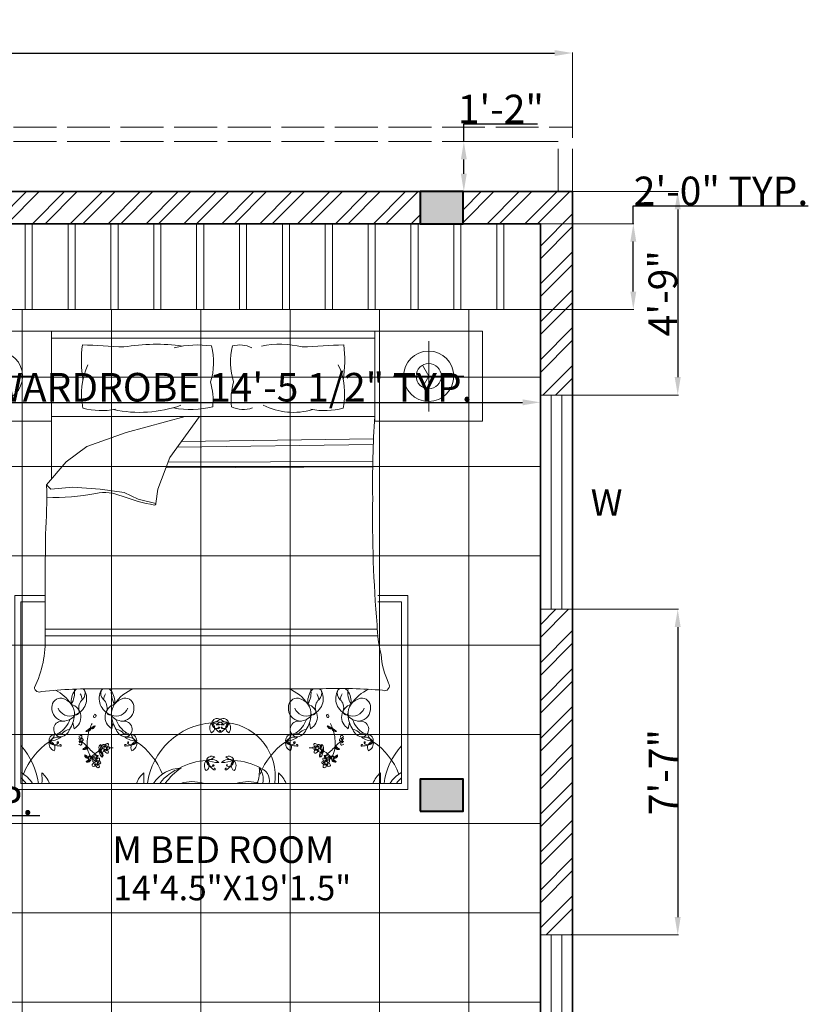
# Model space of a CAD drawing. Units: inches. Extents: x 351 to 1738, y -265 to 286.
# Tile 7 of 38: x 759 to 980, y 10 to 286. Entities that reach past the tile are written whole.
import ezdxf

# ---------------------------------------------------------------- set-up
doc = ezdxf.new("R2010")
doc.units = ezdxf.units.IN
doc.header["$MEASUREMENT"] = 0
doc.linetypes.add('ACAD_ISO02W100', pattern=[15, 12, -3])
for name, color, linetype, lineweight in [('A-ANNO-DIMS', 2, 'Continuous', 18), ('A-ANNO-SYMB', 7, 'Continuous', 18), ('A-AREA-IDEN', 7, 'Continuous', 18), ('A-COLS', 7, 'Continuous', 40), ('A-COLS-PATT', 6, 'Continuous', 13), ('A-FLOR-CASE', 9, 'Continuous', 18), ('A-FLOR-OVHD', 1, 'ACAD_ISO02W100', 18), ('A-FLOR-PATT', 9, 'Continuous', 9), ('A-FURN', 18, 'Continuous', 13), ('A-GLAZ', 4, 'Continuous', 18), ('A-WALL', 7, 'Continuous', 35), ('A-WALL-PATT', 152, 'Continuous', 13)]:
    doc.layers.add(name, color=color, linetype=linetype, lineweight=lineweight)
doc.styles.add('Annotative', font='arial.ttf')
doc.styles.get("Standard").update_dxf_attribs({"font": 'arial.ttf'})
doc.dimstyles.get("Standard").update_dxf_attribs({"dimtxt": 8, "dimasz": 5, "dimexe": 0.18, "dimexo": 0.0625, "dimgap": 0.09, "dimtad": 1, "dimtoh": 1, "dimzin": 0, "dimdsep": 46, "dimlunit": 4, "dimtxsty": 'Standard', "dimcen": 0, "dimclre": 256, "dimadec": 0, "dimazin": 0, "dimtfac": 1, "dimtofl": 0, "dimtmove": 0, "dimatfit": 3, "dimfxl": 1, "dimtolj": 1, "dimtzin": 0, "dimlwe": -1, "dimarcsym": 0})

# ---------------------------------------------------------------- blocks, each defined once
blk = doc.blocks.new('*D2')
at = {"layer": 'A-ANNO-DIMS', "color": 0, "transparency": 16777216}
for p, q in [((382.16, 256.03), (382.16, 276.92)), ((914.16, 256.03), (914.16, 276.92))]:
    blk.add_line(p, q, dxfattribs=at)
at = {"layer": 'A-ANNO-DIMS', "color": 0, "lineweight": -2, "transparency": 16777216}
blk.add_line((387.16, 276.74), (909.16, 276.74), dxfattribs=at)
at = {"layer": 'A-ANNO-DIMS', "color": 0, "transparency": 16777216}
for points in [[(387.16, 277.57), (387.16, 275.91), (382.16, 276.74)], [(909.16, 277.57), (909.16, 275.91), (914.16, 276.74)]]:
    blk.add_solid(points, dxfattribs=at)
at = {"layer": 'Defpoints', "color": 0, "transparency": 16777216}
for p in [(914.16, 276.74), (382.16, 255.96), (914.16, 255.96)]:
    blk.add_point(p, dxfattribs=at)
at = {"layer": 'A-ANNO-DIMS', "color": 0, "transparency": 16777216, "insert": (648.16, 280.83), "char_height": 8, "attachment_point": 5}
blk.add_mtext('\\A1;44\'-4"', dxfattribs=at)
blk = doc.blocks.new('*D4')
at = {"layer": 'A-ANNO-DIMS', "color": 0, "lineweight": -2, "transparency": 16777216}
for p, q in [((883.73, 251.96), (883.73, 256.96)), ((883.73, 256.96), (904.33, 256.96)), ((883.73, 242.96), (883.73, 246.96))]:
    blk.add_line(p, q, dxfattribs=at)
at = {"layer": 'A-ANNO-DIMS', "color": 0, "transparency": 16777216}
for p, q in [((910.09, 251.96), (883.55, 251.96)), ((910.09, 237.96), (883.55, 237.96))]:
    blk.add_line(p, q, dxfattribs=at)
for points in [[(882.9, 246.96), (884.56, 246.96), (883.73, 251.96)], [(882.9, 242.96), (884.56, 242.96), (883.73, 237.96)]]:
    blk.add_solid(points, dxfattribs=at)
at = {"layer": 'Defpoints', "color": 0, "transparency": 16777216}
for p in [(883.73, 251.96), (910.16, 251.96), (910.16, 237.96)]:
    blk.add_point(p, dxfattribs=at)
at = {"layer": 'A-ANNO-DIMS', "color": 0, "transparency": 16777216, "insert": (894.08, 261.07), "char_height": 8, "attachment_point": 5}
blk.add_mtext('\\A1;1\'-2"', dxfattribs=at)
blk = doc.blocks.new('BED-DOUBLE-W-NIGHTSTANDS')
for p, q in [((30.18, 128.33), (30.18, 86.91)), ((15.09, 105.9), (15.09, 125.61)), ((120.72, 126.39), (30.18, 126.39)), ((135.81, 105.9), (135.81, 125.61)), ((24.95, 115.76), (5.23, 115.76)), ((125.95, 115.76), (145.67, 115.76)), ((30.18, 104.48), (120.72, 104.48)), ((120.26, 96.67), (65.46, 95.89)), ((120.32, 98.22), (66.59, 97.46)), ((120.18, 91.92), (62.88, 91.69)), ((120.19, 90.37), (62.29, 90.13)), ((121.41, 44.95), (28.44, 44.95)), ((121.55, 43.07), (28.44, 43.07)), ((106.08, 28.24), (44.82, 28.24)), ((36.54, 17.05), (36.2, 18.75)), ((47.08, 17.05), (47.42, 18.75)), ((102.76, 17.05), (102.43, 18.75)), ((113.31, 17.05), (113.64, 18.75))]:
    blk.add_line(p, q)
for points in [[(30.18, 103.18), (0, 103.18), (0, 128.33), (150.9, 128.33), (150.9, 103.18), (120.72, 103.18), (120.72, 128.33)], [(16.85, 112.71), (15.09, 115.76), (16.85, 118.81)], [(134.05, 118.81), (135.81, 115.76), (134.05, 112.71)], [(71.64, 104.48), (63.37, 92.97), (60, 84.12), (59.39, 80.15), (54.5, 81.37), (50.53, 83.2), (43.81, 84.12), (36.16, 84.73), (30.05, 84.12), (28.83, 85.34), (34.33, 91.75), (40.14, 96.03), (51.14, 100), (67.6, 104.48)], [(121.56, 54.36), (129.93, 54.36), (129.93, 0), (19.92, 0), (19.92, 54.36), (28.45, 54.36)], [(28.45, 52.61), (21.67, 52.61), (21.67, 1.75), (128.18, 1.75), (128.18, 52.61), (121.53, 52.61)]]:
    blk.add_lwpolyline(points)
for points in [[(38.85, 124.57, 0.074897), (39.03, 114.71, -0.472817)], [(74.74, 114.16, 0.14099), (75.04, 124.22, 0.235245)], [(81.19, 114.16, -0.14099), (80.89, 124.22, -0.235245)], [(112.05, 124.57, -0.074897), (111.87, 114.71, 0.472817)], [(28.51, 71.52, 0.001242), (28.44, 42.89, -0.127202), (25.42, 28.62)], [(121.36, 46.14, 0.056112), (122.46, 37.83, 0.095341), (124.58, 29.84)]]:
    blk.add_lwpolyline(points, format="xyb")
for centre, radius in [((15.09, 115.76), 7.04), ((135.81, 115.76), 7.04), ((15.09, 115.76), 3.52), ((135.81, 115.76), 3.52), ((45.25, 11.58), 0.384), ((104.59, 11.58), 0.384), ((42.74, 7.53), 0.384), ((107.11, 7.53), 0.384)]:
    blk.add_circle(centre, radius)
for centre, radius, start, end in [((122.02, 1560.65), 1438.48, 266.68521, 267.14978), ((59.52, 69.97), 54.73, 82.2196, 99.497), ((71.08, 97.62), 26.89, 81.5249, 103.96), ((82.96, 117.05), 7.46, 63.3437, 106.1026), ((94.14, 98.17), 26.53, 76.3427, 101.1841), ((28.88, 1560.65), 1438.48, 272.85022, 273.31479), ((58.07, 110.76), 19.45, 155.1316, 191.7583), ((92.83, 110.76), 19.45, 348.2417, 24.8684), ((56.95, 109.12), 18.49, 354.0129, 15.8293), ((98.98, 109.12), 18.49, 164.1707, 185.9871), ((54.88, 140.71), 35.07, 258.0397, 289.2615), ((97.94, 124.85), 19.21, 243.8761, 286.1746), ((44.23, 126.34), 20.22, 255.1039, 281.0369), ((69.08, 133.05), 26.61, 259.8617, 283.6238), ((83.97, 114.44), 8, 245.0183, 288.5407), ((106.67, 126.34), 20.22, 258.9631, 284.8961), ((391.24, 86.04), 271.14, 176.1, 180.9282), ((-109.53, 81.59), 138.41, 355.8294, 1.553), ((31.41, 138.78), 56.95, 267.4519, 281.3392), ((45.02, 70.89), 12.28, 66.2616, 101.3392), ((69.87, 137.17), 58.52, 250.1194, 259.3383), ((59.05, 80.02), 0.364, 268.8623, 19.7536), ((473.78, 76.18), 353.69, 179.1145, 184.8735), ((26.8, 28.72), 1.39, 183.98, 297.3412), ((43.02, -128.84), 157.09, 89.3433, 95.6887), ((26.22, 17.62), 11.42, 33.6671, 63.2997), ((41.52, 24.41), 5.82, 145.785, 184.7304), ((30.41, 27.13), 6.25, 328.8218, 9.1554), ((38.15, 26.57), 1.82, 120.0293, 142.325), ((35.25, 25.5), 4.81, 289.2822, 29.1751), ((37.38, 26.93), 2.26, 311.5653, 23.8354), ((38.15, 26.57), 1.82, 44.4517, 63.558), ((48.37, 25.5), 4.81, 150.8249, 250.7178), ((46.24, 26.93), 2.26, 156.1646, 228.4347), ((45.47, 26.57), 1.82, 113.229, 135.5483), ((45.47, 26.57), 1.82, 37.675, 66.7144), ((42.1, 24.41), 5.82, 355.2696, 34.215), ((53.21, 27.13), 6.25, 169.7133, 211.1782), ((57.4, 17.62), 11.42, 111.4941, 146.3329), ((92.44, 17.62), 11.42, 33.6671, 68.5059), ((107.75, 24.41), 5.82, 145.785, 184.7304), ((96.63, 27.13), 6.25, 328.8218, 10.2867), ((104.38, 26.57), 1.82, 113.2856, 142.325), ((101.48, 25.5), 4.81, 289.2822, 29.1751), ((104.38, 26.57), 1.82, 44.4517, 66.7144), ((103.61, 26.93), 2.26, 311.5653, 23.8354), ((110.71, -118.52), 146.84, 85.2402, 91.8035), ((114.6, 25.5), 4.81, 150.8249, 250.7178), ((112.47, 26.93), 2.26, 156.1646, 228.4347), ((111.7, 26.57), 1.82, 106.6343, 135.5483), ((111.7, 26.57), 1.82, 37.675, 72.5814), ((108.32, 24.41), 5.82, 355.2696, 34.215), ((119.44, 27.13), 6.25, 169.249, 211.1782), ((123.63, 17.62), 11.42, 113.6453, 146.3329), ((123.44, 29.07), 1.38, 246.5219, 33.8264), ((32.87, 23.1), 2.55, 84.4856, 181.0538), ((32.09, 21.21), 4.54, 355.2933, 76.921), ((40.93, 22.93), 3.09, 131.5653, 195.1471), ((34.52, 24.63), 4.34, 7.436, 29.9149), ((42.69, 22.93), 3.09, 344.8529, 48.4347), ((49.1, 24.63), 4.34, 150.0851, 172.564), ((51.53, 21.21), 4.54, 103.079, 184.7067), ((50.75, 23.1), 2.55, 358.9462, 95.5144), ((99.1, 23.1), 2.55, 84.4856, 181.0538), ((98.32, 21.21), 4.54, 355.2933, 76.921), ((107.16, 22.93), 3.09, 131.5653, 195.1471), ((100.75, 24.63), 4.34, 7.436, 29.9149), ((108.92, 22.93), 3.09, 344.8529, 48.4347), ((115.33, 24.63), 4.34, 150.0851, 172.564), ((117.76, 21.21), 4.54, 103.079, 184.7067), ((116.98, 23.1), 2.55, 358.9462, 95.5144), ((33.91, 22.74), 3.61, 174.9449, 262.8857), ((35.33, 24.1), 3.5, 201.5819, 291.4221), ((34.67, 20.3), 3.75, 299.9085, 73.1337), ((37.04, 21.88), 0.937, 257.3041, 15.1471), ((48.95, 20.3), 3.75, 106.8663, 240.0915), ((46.58, 21.88), 0.937, 164.8529, 282.6959), ((48.29, 24.1), 3.5, 248.5779, 338.4181), ((49.7, 22.74), 3.61, 277.1143, 5.0551), ((100.14, 22.74), 3.61, 174.9449, 262.8857), ((101.56, 24.1), 3.5, 201.5819, 291.4221), ((100.89, 20.3), 3.75, 299.9085, 73.1337), ((103.27, 21.88), 0.937, 257.3041, 15.1471), ((115.18, 20.3), 3.75, 106.8663, 240.0915), ((112.81, 21.88), 0.937, 164.8529, 282.6959), ((114.52, 24.1), 3.5, 248.5779, 338.4181), ((115.93, 22.74), 3.61, 277.1143, 5.0551), ((28.59, 21.91), 7.12, 301.2614, 341.7045), ((33.29, 23.54), 4.38, 272.3591, 324.0401), ((28.53, 21.34), 8.1, 326.2883, 356.5076), ((41.52, 24.41), 5.82, 212.7011, 216.3445), ((42.24, 20.46), 0.291, 102.7051, 280.4384), ((42.21, 20.63), 0.473, 280.4384, 100.4136), ((42.1, 24.41), 5.82, 323.6555, 327.2989), ((50.33, 23.54), 4.38, 215.9599, 267.6409), ((55.09, 21.34), 8.1, 183.4924, 213.7117), ((55.02, 21.91), 7.12, 198.2955, 238.7386), ((76.66, 18.28), 1.63, 63.0274, 163.8037), ((75, 22.1), 3.37, 271.4585, 315.3727), ((78.22, 18.28), 1.63, 16.1963, 116.9726), ((79.87, 22.1), 3.37, 224.6273, 268.5415), ((94.82, 21.91), 7.12, 301.2614, 341.7045), ((99.52, 23.54), 4.38, 272.3591, 324.0401), ((94.76, 21.34), 8.1, 326.2883, 356.5076), ((107.75, 24.41), 5.82, 212.7011, 216.3445), ((107.64, 20.63), 0.473, 79.5864, 259.5616), ((107.6, 20.46), 0.291, 259.5616, 77.2949), ((108.32, 24.41), 5.82, 323.6555, 327.2989), ((116.56, 23.54), 4.38, 215.9599, 267.6409), ((121.32, 21.34), 8.1, 183.4924, 213.7117), ((121.25, 21.91), 7.12, 198.2955, 238.7386), ((33.08, 16.92), 2.26, 80.264, 250.8688), ((32.54, 17.61), 2.83, 265.969, 344.3045), ((35.59, 13.85), 3.01, 96.1662, 141.5825), ((40.58, 15.96), 0.792, 101.3256, 154.4621), ((39.44, 18.65), 2.39, 280.2588, 300.656), ((38.92, 18.64), 2.42, 308.2101, 316.3071), ((40.41, 17.05), 0.724, 278.3432, 4.2869), ((40.01, 17.68), 1.26, 300.656, 332.6341), ((40.96, 16.85), 0.307, 55.7657, 157.4417), ((52.7, 12.86), 12.5, 153.0032, 159.8941), ((41.44, 17.14), 0.307, 84.3784, 186.0543), ((41.15, 18.37), 1.26, 269.1859, 301.164), ((41.52, 17.71), 0.724, 237.5332, 323.4768), ((40.82, 19.78), 2.42, 285.5129, 293.6099), ((42.4, 17.05), 0.792, 87.3579, 140.4944), ((40.57, 19.33), 2.39, 301.164, 321.5612), ((38.63, 19.74), 4.26, 324.6898, 333.4936), ((48.03, 13.85), 3.01, 38.4175, 83.8338), ((51.08, 17.61), 2.83, 195.6955, 274.031), ((50.53, 16.92), 2.26, 289.1312, 99.736), ((76.62, -0.91), 19.71, 94.4623, 172.255), ((76.71, 17.27), 2.19, 137.7873, 219.1145), ((74.23, 17.34), 1.65, 298.5391, 58.3627), ((76.37, 15.9), 3.12, 45.5411, 114.3101), ((79.21, 31.89), 13.79, 252.593, 267.2582), ((76.7, 18.68), 1.61, 177.7585, 283.852), ((79.8, 20.35), 4.98, 198.9159, 238.011), ((78.5, 15.9), 3.12, 65.6899, 134.4589), ((75.66, 31.89), 13.79, 272.7418, 287.407), ((77.04, 17.32), 0.213, 283.852, 219.9245), ((77.29, 16.34), 0.245, 238.011, 71.5592), ((77.33, 16.45), 0.119, 71.5592, 188.0167), ((77.58, 16.34), 0.245, 108.4408, 301.989), ((77.54, 16.45), 0.119, 351.9833, 108.4408), ((77.82, 17.4), 0.128, 320.1909, 256.0209), ((75.07, 20.35), 4.98, 301.989, 341.0841), ((78.18, 18.68), 1.61, 256.148, 2.2415), ((80.65, 17.34), 1.65, 121.6373, 241.4609), ((78.17, 17.27), 2.19, 320.8855, 42.2127), ((77.62, 3.64), 15.25, 352.8636, 81.8197), ((99.31, 16.92), 2.26, 80.264, 250.8688), ((98.77, 17.61), 2.83, 265.969, 344.3045), ((101.82, 13.85), 3.01, 96.1662, 141.5825), ((109.28, 19.33), 2.39, 218.4388, 238.836), ((107.45, 17.05), 0.792, 39.5056, 92.6421), ((111.22, 19.74), 4.26, 206.5064, 215.3102), ((108.33, 17.71), 0.724, 216.5232, 302.4668), ((108.7, 18.37), 1.26, 238.836, 270.8141), ((109.03, 19.78), 2.42, 246.3901, 254.4871), ((97.15, 12.86), 12.5, 20.1059, 26.9968), ((108.41, 17.14), 0.307, 353.9457, 95.6216), ((109.44, 17.05), 0.724, 175.7131, 261.6568), ((108.89, 16.85), 0.307, 22.5583, 124.2343), ((109.84, 17.68), 1.26, 207.3659, 239.344), ((110.93, 18.64), 2.42, 223.6929, 231.7899), ((110.41, 18.65), 2.39, 239.344, 259.7412), ((109.27, 15.96), 0.792, 25.5379, 78.6744), ((117.31, 17.61), 2.83, 195.6955, 274.031), ((114.26, 13.85), 3.01, 38.4175, 83.8338), ((116.76, 16.92), 2.26, 289.1312, 99.736), ((31.17, 13.79), 1.63, 92.9516, 193.728), ((27.83, 16.28), 3.37, 301.3827, 345.2969), ((32.11, 11.59), 3.12, 75.4653, 144.2343), ((26.59, 26.86), 13.79, 282.5173, 297.1824), ((32.62, 14.47), 1.39, 63.9755, 143.2681), ((38.34, 14.46), 0.641, 101.5637, 142.6358), ((37.8, 13.86), 0.384, 273.2768, 86.7232), ((38.25, 14.23), 0.367, 91.1081, 181.8675), ((38.64, 13.49), 0.794, 80.3487, 133.6538), ((37.82, 14.96), 0.924, 288.7263, 352.5032), ((38.49, 12.66), 1.26, 83.0852, 105.7171), ((38.45, 14.92), 0.297, 345.2356, 144.9248), ((38.72, 13.95), 0.331, 317.6792, 80.3487), ((39.99, 20.56), 4.26, 268.3264, 277.1302), ((52.7, 12.86), 12.5, 163.5842, 183.8277), ((51, 14.47), 1.39, 36.7319, 116.0245), ((51.51, 11.59), 3.12, 35.7657, 104.5347), ((57.03, 26.86), 13.79, 242.8176, 257.4827), ((52.45, 13.79), 1.63, 346.272, 87.0484), ((55.79, 16.28), 3.37, 194.7031, 238.6173), ((97.39, 13.79), 1.63, 92.9516, 193.728), ((94.06, 16.28), 3.37, 301.3827, 345.2969), ((98.34, 11.59), 3.12, 75.4653, 144.2343), ((92.82, 26.86), 13.79, 282.5173, 297.1824), ((98.85, 14.47), 1.39, 63.9755, 143.2681), ((97.15, 12.86), 12.5, 356.1723, 16.4158), ((109.86, 20.56), 4.26, 262.8698, 271.6736), ((111.13, 13.95), 0.331, 99.6513, 222.3208), ((111.21, 13.49), 0.794, 46.3462, 99.6513), ((111.4, 14.92), 0.297, 35.0752, 194.7644), ((112.03, 14.96), 0.924, 187.4968, 251.2737), ((111.36, 12.66), 1.26, 74.2829, 96.9148), ((111.6, 14.23), 0.367, 358.1325, 88.8919), ((111.51, 14.46), 0.641, 37.3642, 78.4363), ((112.04, 13.86), 0.384, 93.2768, 266.7232), ((117.23, 14.47), 1.39, 36.7319, 116.0245), ((117.74, 11.59), 3.12, 35.7657, 104.5347), ((123.26, 26.86), 13.79, 242.8176, 257.4827), ((122.02, 16.28), 3.37, 194.7031, 238.6173), ((118.68, 13.79), 1.63, 346.272, 87.0484), ((7, -0.91), 19.71, 7.745, 41.8856), ((40.71, -2.86), 19.71, 124.3865, 158.5908), ((31.71, 12.94), 2.19, 167.7115, 249.0387), ((29.53, 11.76), 1.65, 328.4633, 88.2869), ((32.86, 17.16), 4.98, 228.8402, 267.9352), ((31.01, 14.16), 1.61, 207.6827, 313.7762), ((31.97, 13.15), 0.213, 313.7762, 249.7183), ((32.66, 12.55), 0.119, 101.4834, 217.9409), ((32.69, 12.42), 0.245, 267.9352, 101.4834), ((38.33, 13.15), 0.634, 217.7621, 259.0403), ((39.01, 14), 1.17, 203.4276, 227.6104), ((38.5, 14.15), 0.629, 229.7889, 317.6792), ((37.79, 12.81), 0.893, 355.053, 68.3618), ((38.39, 12.76), 0.295, 232.4737, 355.053), ((29.78, 2.23), 14.33, 43.1541, 52.0459), ((39.68, 10.88), 0.792, 101.3256, 154.4621), ((38.54, 13.57), 2.39, 280.2588, 300.656), ((39.09, 15.48), 4.26, 268.3264, 277.1302), ((38.02, 13.56), 2.42, 308.2101, 316.3071), ((39.51, 11.97), 0.724, 278.3432, 4.2869), ((39.11, 12.61), 1.26, 300.656, 332.6341), ((40.06, 11.77), 0.307, 55.7657, 157.4417), ((46.48, 12.55), 6.27, 184.756, 209.2041), ((55.5, 25.89), 20.62, 222.2412, 232.1744), ((43.25, 11.76), 1.06, 272.8499, 356.1226), ((42.31, 12.15), 1.75, 304.5369, 16.3699), ((42.5, 11.35), 1.03, 321.7607, 7.9252), ((44.74, 11.66), 1.24, 127.3105, 187.9252), ((43.04, 11.8), 1.27, 355.0106, 41.658), ((44.45, 10.86), 0.381, 148.0499, 225.6268), ((47.12, 4.22), 7.52, 113.0501, 113.8477), ((45.15, 10.42), 1.21, 104.7558, 148.0499), ((44.47, 11.29), 0.758, 247.4086, 351.4386), ((44.83, 12.11), 0.524, 126.1046, 271.4281), ((44.77, 12.26), 0.377, 353.7526, 131.7054), ((44.68, 11.26), 0.255, 262.906, 7.132), ((44.42, 11.81), 0.529, 0.0645, 61.1507), ((44.54, 12.26), 0.604, 311.8413, 355.7877), ((45.78, 10.87), 0.634, 151.2196, 259.0403), ((45.79, 12.17), 0.641, 101.5637, 176.365), ((45.7, 11.94), 0.367, 91.1081, 181.8675), ((46.46, 11.71), 1.17, 203.4276, 227.6104), ((46.09, 11.2), 0.794, 80.3487, 133.6538), ((45.95, 11.86), 0.629, 229.7889, 317.6792), ((45.27, 12.68), 0.924, 288.7263, 352.5032), ((45.24, 10.53), 0.893, 355.053, 68.3618), ((45.94, 10.38), 1.26, 83.0852, 105.7171), ((45.9, 12.63), 0.297, 345.2356, 144.9248), ((46.17, 11.66), 0.331, 317.6792, 80.3487), ((47.12, 4.22), 7.52, 87.1071, 94.7585), ((50.93, 12.42), 0.245, 78.5166, 272.0648), ((50.76, 17.16), 4.98, 272.0648, 311.1598), ((50.96, 12.55), 0.119, 322.0591, 78.5166), ((52.61, 14.16), 1.61, 226.2238, 332.3173), ((51.67, 13.23), 0.128, 290.2667, 226.2271), ((54.09, 11.76), 1.65, 91.7131, 211.5367), ((51.9, 12.94), 2.19, 290.9613, 12.2885), ((42.91, -2.86), 19.71, 21.4092, 55.6135), ((106.94, -2.86), 19.71, 124.3865, 158.5908), ((97.94, 12.94), 2.19, 167.7115, 249.0387), ((97.24, 14.16), 1.61, 207.6827, 313.7762), ((99.09, 17.16), 4.98, 228.8402, 267.9352), ((95.76, 11.76), 1.65, 328.4633, 88.2869), ((98.2, 13.15), 0.213, 313.7762, 249.7183), ((98.89, 12.55), 0.119, 101.4834, 217.9409), ((98.92, 12.42), 0.245, 267.9352, 101.4834), ((102.73, 4.22), 7.52, 85.2415, 92.8929), ((103.68, 11.66), 0.331, 99.6513, 222.3208), ((103.9, 11.86), 0.629, 222.3208, 310.2111), ((103.76, 11.2), 0.794, 46.3462, 99.6513), ((103.95, 12.63), 0.297, 35.0752, 194.7644), ((104.58, 12.68), 0.924, 187.4968, 251.2737), ((104.61, 10.53), 0.893, 111.6382, 184.947), ((103.91, 10.38), 1.26, 74.2829, 96.9148), ((104.15, 11.94), 0.367, 358.1325, 88.8919), ((103.38, 11.71), 1.17, 312.3896, 336.5724), ((104.06, 12.17), 0.641, 3.635, 78.4363), ((104.07, 10.87), 0.634, 280.9597, 28.7804), ((105.38, 11.29), 0.758, 188.5614, 292.5914), ((105.08, 12.26), 0.377, 48.2946, 186.2474), ((105.3, 12.26), 0.604, 184.2123, 228.1587), ((105.43, 11.81), 0.529, 118.8493, 179.9355), ((105.16, 11.26), 0.255, 172.868, 277.094), ((105.02, 12.11), 0.524, 268.5719, 53.8954), ((104.7, 10.42), 1.21, 31.9501, 75.2442), ((106.81, 11.8), 1.27, 138.342, 184.9894), ((106.6, 11.76), 1.06, 183.8774, 267.1501), ((102.73, 4.22), 7.52, 66.1523, 66.9499), ((105.4, 10.86), 0.381, 314.3732, 31.9501), ((107.53, 12.15), 1.75, 163.6301, 235.4631), ((105.1, 11.66), 1.24, 352.0748, 52.6895), ((107.35, 11.35), 1.03, 172.0748, 218.2393), ((94.35, 25.89), 20.62, 307.8256, 317.7588), ((103.37, 12.55), 6.27, 330.7959, 355.244), ((110.34, 11.97), 0.724, 175.7131, 261.6568), ((120.07, 2.23), 14.33, 127.9541, 136.8459), ((109.79, 11.77), 0.307, 22.5583, 124.2343), ((110.74, 12.61), 1.26, 207.3659, 239.344), ((111.83, 13.56), 2.42, 223.6929, 231.7899), ((111.31, 13.57), 2.39, 239.344, 259.7412), ((110.76, 15.48), 4.26, 262.8698, 271.6736), ((110.17, 10.88), 0.792, 25.5379, 78.6744), ((111.35, 14.15), 0.629, 222.3208, 310.2111), ((112.06, 12.81), 0.893, 111.6382, 184.947), ((111.46, 12.76), 0.295, 184.947, 307.5263), ((110.83, 14), 1.17, 312.3896, 336.5724), ((111.52, 13.15), 0.634, 280.9597, 322.2379), ((117.16, 12.42), 0.245, 78.5166, 272.0648), ((116.99, 17.16), 4.98, 272.0648, 311.1598), ((117.18, 12.55), 0.119, 322.0591, 78.5166), ((118.84, 14.16), 1.61, 226.2238, 332.3173), ((117.9, 13.23), 0.128, 290.2667, 226.2271), ((120.32, 11.76), 1.65, 91.7131, 211.5367), ((118.13, 12.94), 2.19, 290.9613, 12.2885), ((109.14, -2.86), 19.71, 21.4092, 55.6135), ((142.85, -0.91), 19.71, 138.1144, 172.255), ((39.94, 9.49), 0.429, 146.8636, 236.9021), ((45.99, 18.94), 11.23, 235.1882, 238.8844), ((40.68, 10.11), 1.16, 199.4799, 267.6828), ((40.55, 9.68), 1, 212.8155, 277.3992), ((39.97, 9.01), 1.16, 266.9701, 338.2913), ((40.42, 9.71), 0.444, 238.8844, 314.2646), ((40.33, 8.72), 1, 280.3057, 17.1958), ((40.24, 8.61), 0.444, 306.3746, 21.7548), ((40.96, 8.9), 0.335, 19.3605, 201.7548), ((40.97, 9.16), 0.335, 311.8703, 134.2646), ((47.27, 6.1), 6.69, 153.7819, 158.2913), ((41.94, 10.67), 1.75, 247.2305, 319.0635), ((41.36, 10.08), 1.03, 264.4544, 310.6188), ((46.48, 12.55), 6.27, 214.0033, 222.4917), ((42.12, 9.68), 1.06, 218.3208, 298.8162), ((47.12, 4.22), 7.52, 120.544, 139.818), ((42.32, 8.06), 0.524, 126.1046, 271.4281), ((42.26, 8.21), 0.377, 353.7526, 131.7054), ((42.84, 8.36), 1.24, 70.0041, 130.6188), ((42.04, 9.87), 1.27, 297.7043, 344.3516), ((43.27, 8.12), 0.641, 101.5637, 176.365), ((42.76, 8.63), 0.924, 288.7263, 352.5032), ((43.39, 8.58), 0.297, 345.2356, 144.9248), ((42.71, 9.86), 1.03, 8.7227, 54.8872), ((42.77, 9.04), 1.75, 0.278, 72.111), ((43.55, 9.68), 1.06, 20.5253, 88.5375), ((44.96, 10.21), 1.24, 188.7227, 249.3375), ((43.37, 9.59), 1.27, 334.9899, 21.6373), ((45.84, 10.48), 0.295, 232.4737, 355.053), ((75.15, 7.73), 1.63, 63.0274, 163.8037), ((73.5, 11.55), 3.37, 271.4585, 315.3727), ((74.86, 5.35), 3.12, 45.5411, 114.3101), ((80.01, 5.35), 3.12, 65.6899, 134.4589), ((79.73, 7.73), 1.63, 16.1963, 116.9726), ((81.38, 11.55), 3.37, 224.6273, 268.5415), ((104.01, 10.48), 0.295, 184.947, 307.5263), ((106.48, 9.59), 1.27, 158.3627, 205.0101), ((106.3, 9.68), 1.06, 91.4625, 159.4747), ((107.08, 9.04), 1.75, 107.889, 179.722), ((104.89, 10.21), 1.24, 290.6625, 351.2773), ((107.13, 9.86), 1.03, 125.1128, 171.2773), ((106.46, 8.58), 0.297, 35.0752, 194.7644), ((107.09, 8.63), 0.924, 187.4968, 251.2737), ((102.73, 4.22), 7.52, 40.182, 59.456), ((107.01, 8.36), 1.24, 49.3812, 109.9959), ((107.91, 10.67), 1.75, 220.9365, 292.7695), ((107.81, 9.87), 1.27, 195.6484, 242.2957), ((106.58, 8.12), 0.641, 3.635, 78.4363), ((107.59, 8.21), 0.377, 48.2946, 186.2474), ((107.73, 9.68), 1.06, 241.1838, 321.6792), ((107.53, 8.06), 0.524, 268.5719, 53.8954), ((108.49, 10.08), 1.03, 229.3812, 275.5456), ((103.37, 12.55), 6.27, 317.5083, 325.9967), ((109.52, 8.72), 1, 162.8042, 259.6943), ((108.88, 9.16), 0.335, 45.7354, 228.1297), ((108.88, 8.9), 0.335, 338.2452, 160.6395), ((102.58, 6.1), 6.69, 21.7087, 26.2181), ((109.88, 9.01), 1.16, 201.7087, 273.0299), ((109.42, 9.71), 0.444, 225.7354, 301.1156), ((109.61, 8.61), 0.444, 158.2452, 233.6254), ((109.3, 9.68), 1, 262.6008, 327.1845), ((109.17, 10.11), 1.16, 272.3172, 340.5201), ((103.85, 18.94), 11.23, 301.1156, 304.8118), ((109.9, 9.49), 0.429, 303.0979, 33.1364), ((33.85, 17.3), 11.23, 302.6784, 306.3746), ((40.26, 8.09), 0.429, 214.3538, 304.3923), ((41.93, 6.81), 0.381, 148.0499, 225.6268), ((42.64, 6.37), 1.21, 104.7558, 148.0499), ((41.96, 7.24), 0.758, 247.4086, 351.4386), ((42.17, 7.2), 0.255, 262.906, 7.132), ((41.9, 7.76), 0.529, 0.0645, 61.1507), ((42.03, 8.21), 0.604, 311.8413, 355.7877), ((43.26, 6.82), 0.634, 151.2196, 259.0403), ((43.19, 7.89), 0.367, 91.1081, 181.8675), ((43.95, 7.66), 1.17, 203.4276, 227.6104), ((43.58, 7.15), 0.794, 80.3487, 133.6538), ((43.44, 7.81), 0.629, 229.7889, 317.6792), ((42.73, 6.48), 0.893, 355.053, 68.3618), ((43.43, 6.33), 1.26, 83.0852, 105.7171), ((43.32, 6.43), 0.295, 232.4737, 355.053), ((43.66, 7.61), 0.331, 317.6792, 80.3487), ((66.74, -3.55), 9.6, 91.272, 146.5383), ((70.19, -5.34), 11.97, 107.8504, 143.6964), ((76.48, -8.7), 17.8, 124.0123, 144.053), ((75.11, -11.46), 19.71, 94.4623, 117.4146), ((75.2, 6.72), 2.19, 137.7873, 219.1145), ((72.72, 6.78), 1.65, 298.5391, 58.3627), ((78.3, 9.8), 4.98, 198.9159, 238.011), ((77.71, 21.34), 13.79, 252.593, 267.2582), ((75.19, 8.12), 1.61, 177.7585, 283.852), ((75.53, 6.76), 0.213, 283.852, 219.9245), ((75.79, 5.78), 0.245, 238.011, 71.5592), ((75.83, 5.9), 0.119, 71.5592, 188.0167), ((77.17, 21.34), 13.79, 272.7418, 287.407), ((79.09, 5.78), 0.245, 108.4408, 301.989), ((79.05, 5.9), 0.119, 351.9833, 108.4408), ((79.33, 6.85), 0.128, 320.1909, 256.0209), ((76.58, 9.8), 4.98, 301.989, 341.0841), ((79.69, 8.12), 1.61, 256.148, 2.2415), ((82.16, 6.78), 1.65, 121.6373, 241.4609), ((79.68, 6.72), 2.19, 320.8855, 42.2127), ((79.76, -11.46), 19.71, 62.5854, 85.5377), ((79.59, 5.04), 8.82, 338.117, 6.6195), ((87.68, 2.58), 3.54, 346.3898, 79.0739), ((85.02, 3.07), 4.47, 342.8609, 41.9049), ((106.19, 7.61), 0.331, 99.6513, 222.3208), ((106.41, 7.81), 0.629, 222.3208, 310.2111), ((106.27, 7.15), 0.794, 46.3462, 99.6513), ((107.12, 6.48), 0.893, 111.6382, 184.947), ((106.52, 6.43), 0.295, 184.947, 307.5263), ((106.42, 6.33), 1.26, 74.2829, 96.9148), ((106.66, 7.89), 0.367, 358.1325, 88.8919), ((105.9, 7.66), 1.17, 312.3896, 336.5724), ((106.58, 6.82), 0.634, 280.9597, 28.7804), ((107.89, 7.24), 0.758, 188.5614, 292.5914), ((107.82, 8.21), 0.604, 184.2123, 228.1587), ((107.94, 7.76), 0.529, 118.8493, 179.9355), ((107.68, 7.2), 0.255, 172.868, 277.094), ((107.21, 6.37), 1.21, 31.9501, 75.2442), ((107.91, 6.81), 0.381, 314.3732, 31.9501), ((116, 17.3), 11.23, 233.6254, 237.3216), ((109.59, 8.09), 0.429, 235.6077, 325.6462), ((16.88, -3.55), 9.6, 33.4617, 60.1116), ((13.43, -5.34), 11.97, 36.3036, 46.4814), ((22.26, -1.32), 8.01, 22.5547, 48.9546), ((0.31, 2.98), 27.26, 357.4081, 3.6519), ((61.36, -1.32), 8.01, 131.0454, 157.4453), ((83.31, 2.98), 27.26, 176.3481, 182.5919), ((66.54, 2.98), 27.26, 357.4081, 3.6519), ((88.49, -1.32), 8.01, 22.5547, 48.9546), ((127.59, -1.32), 8.01, 131.0454, 157.4453), ((149.54, 2.98), 27.26, 176.3481, 182.5919), ((132.97, -3.55), 9.6, 119.8884, 146.5383), ((136.42, -5.34), 11.97, 133.5186, 143.6964), ((69.6, -8.61), 10.84, 73.5431, 107.0202), ((73.9, -14.2), 16.02, 94.3787, 95.6357), ((82.34, -25.17), 28.63, 109.7217, 109.9028), ((85.27, -8.61), 10.84, 72.9798, 106.4569), ((80.98, -14.2), 16.02, 84.3643, 85.6213), ((72.54, -25.17), 28.63, 70.0972, 70.2783)]:
    blk.add_arc(centre, radius, start, end)
blk = doc.blocks.new('WARDROBE-PANELLED')
for p, q in [((5.27, 24), (5.27, 0)), ((7.27, 24), (7.27, 0)), ((17.27, 24), (17.27, 0)), ((19.27, 24), (19.27, 0)), ((29.27, 24), (29.27, 0)), ((31.27, 24), (31.27, 0)), ((41.27, 24), (41.27, 0)), ((43.27, 24), (43.27, 0)), ((53.27, 24), (53.27, 0)), ((55.27, 24), (55.27, 0)), ((65.27, 24), (65.27, 0)), ((67.27, 24), (67.27, 0)), ((77.27, 24), (77.27, 0)), ((79.27, 24), (79.27, 0)), ((89.27, 24), (89.27, 0)), ((91.27, 24), (91.27, 0)), ((101.27, 24), (101.27, 0)), ((103.27, 24), (103.27, 0)), ((113.27, 24), (113.27, 0)), ((115.27, 24), (115.27, 0)), ((125.27, 24), (125.27, 0)), ((127.27, 24), (127.27, 0)), ((137.27, 24), (137.27, 0)), ((139.27, 24), (139.27, 0)), ((149.27, 24), (149.27, 0)), ((151.27, 24), (151.27, 0)), ((161.27, 24), (161.27, 0)), ((163.27, 24), (163.27, 0)), ((0, 0), (173.5, 0))]:
    blk.add_line(p, q)
blk = doc.blocks.new('COL-9x12')
blk.add_lwpolyline([(0, 12), (0, 0), (9, 0), (9, 12)], close=True)
blk = doc.blocks.new('WIN-60')
for p, q in [((0, 6), (60, 6)), ((0, 3), (60, 3))]:
    blk.add_line(p, q)
blk.add_lwpolyline([(60, 0), (60, 9), (0, 9), (0, 0)], close=True)
blk = doc.blocks.new('*D40')
at = {"layer": 'A-ANNO-DIMS', "transparency": 16777216}
for p, q in [((654.45, 65.99), (654.45, 63.04)), ((673.33, 65.99), (673.33, 63.04))]:
    blk.add_line(p, q, dxfattribs=at)
at = {"layer": 'A-ANNO-DIMS', "color": 0, "lineweight": -2, "transparency": 16777216}
for p, q in [((659.45, 63.22), (668.33, 63.22)), ((673.33, 63.22), (765.05, 63.22))]:
    blk.add_line(p, q, dxfattribs=at)
at = {"layer": 'A-ANNO-DIMS', "color": 0, "transparency": 16777216}
for points in [[(659.45, 64.06), (659.45, 62.39), (654.45, 63.22)], [(668.33, 64.06), (668.33, 62.39), (673.33, 63.22)]]:
    blk.add_solid(points, dxfattribs=at)
at = {"layer": 'Defpoints', "color": 0, "transparency": 16777216}
for p in [(654.45, 66.05), (673.33, 66.05), (673.33, 63.22)]:
    blk.add_point(p, dxfattribs=at)
at = {"layer": 'A-ANNO-DIMS', "color": 0, "transparency": 16777216, "insert": (721.69, 67.45), "char_height": 8, "attachment_point": 5}
blk.add_mtext('\\A1;CHAIR 1\'-7" TYP.', dxfattribs=at)
blk = doc.blocks.new('*D48')
at = {"layer": 'A-ANNO-DIMS', "transparency": 16777216}
for p, q in [((731.66, 204.9), (731.66, 178.76)), ((905.16, 204.9), (905.16, 178.76))]:
    blk.add_line(p, q, dxfattribs=at)
at = {"layer": 'A-ANNO-DIMS', "color": 0, "lineweight": -2, "transparency": 16777216}
blk.add_line((736.66, 178.94), (900.16, 178.94), dxfattribs=at)
at = {"layer": 'A-ANNO-DIMS', "color": 0, "transparency": 16777216}
for points in [[(736.66, 179.77), (736.66, 178.1), (731.66, 178.94)], [(900.16, 179.77), (900.16, 178.1), (905.16, 178.94)]]:
    blk.add_solid(points, dxfattribs=at)
at = {"layer": 'Defpoints', "color": 0, "transparency": 16777216}
for p in [(731.66, 204.96), (905.16, 204.96), (905.16, 178.94)]:
    blk.add_point(p, dxfattribs=at)
at = {"layer": 'A-ANNO-DIMS', "color": 0, "transparency": 16777216, "insert": (818.41, 183.17), "char_height": 8, "attachment_point": 5}
blk.add_mtext('\\A1;WARDROBE 14\'-5 1/2" TYP.', dxfattribs=at)
blk = doc.blocks.new('*D49')
at = {"layer": 'A-ANNO-DIMS', "color": 0, "lineweight": -2, "transparency": 16777216}
for p, q in [((931.18, 228.96), (931.18, 233.96)), ((931.18, 233.96), (980.17, 233.96)), ((931.18, 209.96), (931.18, 223.96))]:
    blk.add_line(p, q, dxfattribs=at)
at = {"layer": 'A-ANNO-DIMS', "transparency": 16777216}
for p, q in [((905.22, 228.96), (931.36, 228.96)), ((905.22, 204.96), (931.36, 204.96))]:
    blk.add_line(p, q, dxfattribs=at)
at = {"layer": 'A-ANNO-DIMS', "color": 0, "transparency": 16777216}
for points in [[(930.35, 223.96), (932.01, 223.96), (931.18, 228.96)], [(930.35, 209.96), (932.01, 209.96), (931.18, 204.96)]]:
    blk.add_solid(points, dxfattribs=at)
at = {"layer": 'Defpoints', "color": 0, "transparency": 16777216}
for p in [(905.16, 228.96), (931.18, 228.96), (905.16, 204.96)]:
    blk.add_point(p, dxfattribs=at)
at = {"layer": 'A-ANNO-DIMS', "color": 0, "transparency": 16777216, "insert": (955.72, 238.14), "char_height": 8, "attachment_point": 5}
blk.add_mtext('\\A1;2\'-0" TYP.', dxfattribs=at)
blk = doc.blocks.new('*D59')
at = {"layer": 'A-ANNO-DIMS', "transparency": 16777216}
for p, q in [((914.22, 237.96), (943.79, 237.96)), ((914.22, 180.99), (943.79, 180.99))]:
    blk.add_line(p, q, dxfattribs=at)
at = {"layer": 'A-ANNO-DIMS', "color": 0, "lineweight": -2, "transparency": 16777216}
blk.add_line((943.61, 232.96), (943.61, 185.99), dxfattribs=at)
at = {"layer": 'A-ANNO-DIMS', "color": 0, "transparency": 16777216}
for points in [[(942.77, 232.96), (944.44, 232.96), (943.61, 237.96)], [(942.77, 185.99), (944.44, 185.99), (943.61, 180.99)]]:
    blk.add_solid(points, dxfattribs=at)
at = {"layer": 'Defpoints', "color": 0, "transparency": 16777216}
for p in [(914.16, 237.96), (914.16, 180.99), (943.61, 180.99)]:
    blk.add_point(p, dxfattribs=at)
at = {"layer": 'A-ANNO-DIMS', "color": 0, "transparency": 16777216, "insert": (939.43, 209.48), "char_height": 8, "attachment_point": 5, "rotation": 90}
blk.add_mtext('\\A1;4\'-9"', dxfattribs=at)
blk = doc.blocks.new('*D60')
at = {"layer": 'A-ANNO-DIMS', "transparency": 16777216}
for p, q in [((914.22, 120.99), (943.79, 120.99)), ((914.22, 29.81), (943.79, 29.81))]:
    blk.add_line(p, q, dxfattribs=at)
at = {"layer": 'A-ANNO-DIMS', "color": 0, "lineweight": -2, "transparency": 16777216}
blk.add_line((943.61, 115.99), (943.61, 34.81), dxfattribs=at)
at = {"layer": 'A-ANNO-DIMS', "color": 0, "transparency": 16777216}
for points in [[(942.77, 115.99), (944.44, 115.99), (943.61, 120.99)], [(942.77, 34.81), (944.44, 34.81), (943.61, 29.81)]]:
    blk.add_solid(points, dxfattribs=at)
at = {"layer": 'Defpoints', "color": 0, "transparency": 16777216}
for p in [(914.16, 120.99), (914.16, 29.81), (943.61, 29.81)]:
    blk.add_point(p, dxfattribs=at)
at = {"layer": 'A-ANNO-DIMS', "color": 0, "transparency": 16777216, "insert": (939.52, 75.4), "char_height": 8, "attachment_point": 5, "rotation": 90}
blk.add_mtext('\\A1;7\'-7"', dxfattribs=at)

msp = doc.modelspace()

# ---------------------------------------------------------------- hatches: boundary and pattern name
at = {"layer": 'A-COLS-PATT'}
h = msp.add_hatch(color=256, dxfattribs=at)
h.dxf.hatch_style = 1
h.paths.add_polyline_path([(460.155, 237.963), (451.155, 237.963), (451.155, 228.963), (460.155, 228.963)])
h.paths.add_polyline_path([(463.155, 237.963), (460.155, 237.963), (460.155, 228.963), (463.155, 228.963)])
h.paths.add_polyline_path([(391.155, 255.963), (382.155, 255.963), (382.155, 243.963), (391.155, 243.963)])
h.paths.add_polyline_path([(391.155, 210.963), (382.155, 210.963), (382.155, 198.963), (391.155, 198.963)])
h.paths.add_polyline_path([(391.155, -45.037), (382.155, -45.037), (382.155, -57.037), (391.155, -57.037)])
h.paths.add_polyline_path([(460.155, -45.037), (451.155, -45.037), (451.155, -57.037), (460.155, -57.037)])
h.paths.add_polyline_path([(460.155, -161.037), (451.155, -161.037), (451.155, -164.037), (451.155, -173.037), (460.155, -173.037)])
h.paths.add_polyline_path([(391.155, -161.037), (382.155, -161.037), (382.155, -173.037), (391.155, -173.037)])
h.paths.add_polyline_path([(596, -164.037), (584, -164.037), (584, -173.037), (596, -173.037)])
h.paths.add_polyline_path([(596, -50), (584, -50), (584, -59), (596, -59)])
h.paths.add_polyline_path([(596.155, 73.463), (592.155, 73.463), (592.155, 64.463), (596.155, 64.463)])
h.paths.add_polyline_path([(592.155, 73.463), (584.155, 73.463), (584.155, 64.463), (592.155, 64.463)])
h.paths.add_polyline_path([(596.155, 237.963), (584.155, 237.963), (584.155, 228.963), (596.155, 228.963)])
h.paths.add_polyline_path([(739.655, 237.963), (727.655, 237.963), (727.655, 228.963), (739.655, 228.963)])
h.paths.add_polyline_path([(883.515, 237.963), (871.515, 237.963), (871.515, 228.963), (883.515, 228.963)])
h.paths.add_polyline_path([(883.515, 73.463), (871.515, 73.463), (871.515, 64.463), (883.515, 64.463)])
h.paths.add_polyline_path([(731.655, 73.463), (727.655, 73.463), (727.655, 64.463), (731.655, 64.463)])
h.paths.add_polyline_path([(739.515, 73.463), (731.655, 73.463), (731.655, 64.463), (739.515, 64.463)])
h.paths.add_polyline_path([(883.515, -53.037), (871.515, -53.037), (871.515, -57.037), (883.515, -57.037)])
h.paths.add_polyline_path([(883.515, -48.037), (871.515, -48.037), (871.515, -53.037), (883.515, -53.037)])
h.paths.add_polyline_path([(739.515, -48.037), (727.515, -48.037), (727.515, -56.5), (727.516, -57.037), (739.515, -57.037)])
h.paths.add_polyline_path([(883.515, -164.037), (871.515, -164.037), (871.515, -173.037), (883.515, -173.037)])
at = {"layer": 'A-FLOR-PATT', "transparency": 33554559}
h = msp.add_hatch(dxfattribs=at)
h.set_pattern_fill('ANSI37', color=256, scale=200, angle=45)
h.set_pattern_definition([(90, (460.077, -164.037), (-25, 0), []), (180, (460.077, -164.037), (-4e-15, -25), [])])
h.paths.add_polyline_path([(727.516, -57.037), (727.515, -57.037), (727.515, -56.5), (727.5, -45), (727.5, -3.5), (727.501, -2.537), (725.797, -2.537), (725.797, -3.037), (721.988, -3.037), (721.988, -2.537), (717.916, -2.537), (717.916, -3.037), (714.106, -3.037), (714.106, -2.537), (710.487, -2.537), (710.487, -3.037), (706.677, -3.037), (706.677, -2.537), (702.965, -2.537), (702.965, -3.037), (699.155, -3.037), (699.155, -2.537), (694.965, -2.537), (694.965, -3.037), (691.155, -3.037), (691.155, -2.537), (679.655, -2.537), (678.797, -2.537), (677.776, -2.537), (676.723, -2.537), (652.655, -2.537), (651.799, -2.537), (650.778, -2.537), (649.725, -2.537), (625.877, -2.537), (624.879, -2.537), (623.857, -2.537), (622.804, -2.537), (596.155, -2.537), (596.155, -3.537), (460.155, -3.537), (460.155, -81.037), (460.077, -99.07), (460.077, -133.967), (460.155, -152.037), (460.155, -164.037), (485.277, -164.037), (545.277, -164.037), (727.655, -164.037)])
h.paths.add_polyline_path([(584, -59), (584, -50), (596, -50), (596, -59)], flags=16)
h.paths.add_polyline_path([(905.155, 204.963), (731.655, 204.963), (731.655, 73.463), (739.515, 73.463), (739.515, 64.463), (731.655, 64.463), (731.655, -3.5), (727.655, -3.5), (727.655, -3.537), (727.5, -45), (731.655, -45), (731.655, -48.037), (739.515, -48.037), (739.515, -53.037), (754, -53.037), (754, -57.037), (748.655, -57.037), (748.655, -147.037), (815.655, -147.037), (815.655, -138.5), (819.655, -138.5), (819.655, -102.5), (815.655, -102.5), (815.655, -57.037), (790, -57.037), (790, -53.037), (871.515, -53.037), (871.515, -48.037), (883.515, -48.037), (883.515, -53.037), (905.155, -53.037)])
h.paths.add_polyline_path([(871.515, 64.463), (871.515, 73.463), (883.515, 73.463), (883.515, 64.463)], flags=16)
h.paths.add_polyline_path([(727.655, 64.463), (685.515, 64.463), (685.515, 186.963), (638.155, 186.963), (638.155, 88.463), (596.155, 88.463), (596.155, 64.463), (584.155, 64.463), (584.155, 73.463), (592.155, 73.463), (592.155, 205.963), (574, 205.963), (574, 209.963), (538, 209.963), (538, 205.963), (536.5, 205.963), (536.5, 180), (489.5, 180), (489.5, 68.655), (460.155, 68.655), (460.155, 64.463), (536.155, 64.463), (536.155, 48.463), (532.155, 48.463), (532.155, 60.463), (460.155, 60.463), (460.155, 0.463), (532.155, 0.463), (532.155, 12.463), (536.155, 12.463), (536.155, 0.463), (596.155, 0.463), (596.155, -0.537), (622.655, -0.537), (623.655, -0.537), (624.655, -0.537), (625.655, -0.537), (649.655, -0.537), (650.576, -0.537), (651.576, -0.537), (652.576, -0.537), (676.655, -0.537), (677.574, -0.537), (678.574, -0.537), (679.574, -0.537), (691.155, -0.537), (691.155, -0.037), (694.965, -0.037), (694.965, -0.537), (699.155, -0.537), (699.155, -0.037), (702.965, -0.037), (702.965, -0.537), (706.677, -0.537), (706.677, -0.037), (710.487, -0.037), (710.487, -0.537), (714.106, -0.537), (714.106, -0.037), (717.916, -0.037), (717.916, -0.537), (721.988, -0.537), (721.988, -0.037), (725.797, -0.037), (725.797, -0.537), (727.655, -0.537)])
h.paths.add_polyline_path([(485.401, 6.538), (461.783, 6.538), (461.783, 51.327), (485.401, 51.327)], flags=16)
h.paths.add_polyline_path([(483.401, 8.538), (463.783, 8.538), (463.783, 49.327), (483.401, 49.327)], flags=0)
h.paths.add_polyline_path([(476.907, 30.5), (476.907, 29.5), (476.907, 26), (475.907, 26), (475.907, 29.5), (474.449, 29.5), (474.449, 26), (473.449, 26), (470.5, 26), (470.5, 27), (473.449, 27), (473.449, 29.5), (470.5, 29.5), (470.5, 32.758), (471.5, 32.758), (471.5, 30.5), (473.407, 30.5), (473.407, 32.897), (473.407, 33.897), (476.907, 33.897), (476.907, 32.897), (474.407, 32.897), (474.407, 30.5)], flags=0)
at = {"layer": 'A-WALL-PATT'}
h = msp.add_hatch(dxfattribs=at)
h.set_pattern_fill('ANSI32', color=256, scale=20)
h.set_pattern_definition([(45, (382.155, -173.037), (-5.3033, 5.3033), []), (45, (385.691, -173.037), (-5.3033, 5.3033), [])])
h.paths.add_polyline_path([(391.155, -57.037), (382.155, -57.037), (382.155, -81.037), (391.155, -81.037)])
h.paths.add_polyline_path([(391.155, 198.963), (382.155, 198.963), (382.155, -45.037), (391.155, -45.037)])
h.paths.add_polyline_path([(391.155, 243.963), (382.155, 243.963), (382.155, 237.963), (382.155, 210.963), (391.155, 210.963)])
h.paths.add_polyline_path([(460.155, 255.963), (391.155, 255.963), (391.155, 246.963), (451.155, 246.963), (451.155, 237.963), (460.155, 237.963), (460.155, 251.963)])
h.paths.add_polyline_path([(404.155, 207.963), (391.155, 207.963), (391.155, 198.963), (404.155, 198.963)])
h.paths.add_polyline_path([(451.155, 207.963), (440.155, 207.963), (440.155, 198.963), (451.155, 198.963)])
h.paths.add_polyline_path([(460.155, 228.963), (451.155, 228.963), (451.155, 74.963), (460.155, 74.963), (460.155, 97.5)])
h.paths.add_polyline_path([(460.155, 60.463), (532.155, 60.463), (532.155, 48.463), (536.155, 48.463), (536.155, 64.463), (460.155, 64.463), (460.155, 62.963), (451.155, 62.963), (451.155, 46.258), (460.155, 46.258)])
h.paths.add_polyline_path([(460.155, -3.537), (596.155, -3.537), (596.155, 0.463), (536.155, 0.463), (536.155, 12.463), (532.155, 12.463), (532.155, 0.463), (460.155, 0.463), (460.155, 10.258), (451.155, 10.258), (451.155, -45.037), (460.155, -45.037)])
h.paths.add_polyline_path([(460.155, -57.037), (451.155, -57.037), (451.155, -81.037), (460.155, -81.037)])
h.paths.add_polyline_path([(460.155, -152.037), (451.155, -152.037), (451.155, -161.037), (460.155, -161.037)])
h.paths.add_polyline_path([(485.277, -164.037), (460.155, -164.037), (460.155, -164.5), (460.155, -173.037), (485.277, -173.037)])
h.paths.add_polyline_path([(584, -164.037), (545.277, -164.037), (545.277, -173.037), (584, -173.037)])
h.paths.add_polyline_path([(631.58, -164.037), (596, -164.037), (596, -173.037), (631.58, -173.037)])
h.paths.add_polyline_path([(871.515, -164.037), (819.655, -164.037), (819.655, -138.5), (815.655, -138.5), (815.655, -164.037), (691.58, -164.037), (691.58, -173.037), (871.515, -173.037)])
h.paths.add_polyline_path([(731.655, -57.037), (727.516, -57.037), (727.655, -164.037), (731.655, -164.037)])
h.paths.add_polyline_path([(914.155, -138), (905.155, -138), (905.155, -164.037), (883.515, -164.037), (883.515, -173.037), (914.155, -173.037)])
h.paths.add_polyline_path([(914.155, -30.189), (905.155, -30.189), (905.155, -53.037), (883.515, -53.037), (883.515, -57.037), (905.155, -57.037), (905.155, -102), (914.155, -102)])
h.paths.add_polyline_path([(871.515, -53.037), (790, -53.037), (790, -57.037), (815.655, -57.037), (815.655, -102.5), (819.655, -102.5), (819.655, -57.037), (871.515, -57.037)])
h.paths.add_polyline_path([(914.155, 120.993), (905.155, 120.993), (905.155, 29.811), (914.155, 29.811)])
h.paths.add_polyline_path([(731.655, 64.463), (727.655, 64.463), (727.655, -3.5), (731.655, -3.5)])
h.paths.add_polyline_path([(481.5, 209.963), (460.155, 209.963), (460.155, 205.963), (481.5, 205.963)])
h.paths.add_polyline_path([(538, 209.963), (517.5, 209.963), (517.5, 205.963), (538, 205.963)])
h.paths.add_polyline_path([(592.155, 209.963), (574, 209.963), (574, 205.963), (592.155, 205.963)])
h.paths.add_polyline_path([(596.155, 228.963), (592.155, 228.963), (592.155, 73.463), (596.155, 73.463)])
h.paths.add_polyline_path([(614, 237.963), (596.155, 237.963), (596.155, 228.963), (614, 228.963)])
h.paths.add_polyline_path([(677, 237.963), (650, 237.963), (650, 228.963), (677, 228.963)])
h.paths.add_polyline_path([(727.655, 237.963), (713, 237.963), (713, 228.963), (727.655, 228.963)])
h.paths.add_polyline_path([(871.515, 237.963), (739.655, 237.963), (739.655, 228.963), (871.515, 228.963)])
h.paths.add_polyline_path([(731.655, 228.963), (727.655, 228.963), (727.655, 73.463), (731.655, 73.463)])
h.paths.add_polyline_path([(914.155, 237.963), (883.515, 237.963), (883.515, 228.963), (905.155, 228.963), (905.155, 180.993), (914.155, 180.993)])

# ---------------------------------------------------------------- linework, layer by layer
at = {"layer": 'A-FLOR-OVHD'}
for p, q in [((592.655, 255.963), (914.155, 255.963)), ((914.155, 237.963), (914.155, 255.963)), ((592.655, 251.963), (910.155, 251.963)), ((910.155, 237.963), (910.155, 251.963))]:
    msp.add_line(p, q, dxfattribs=at)
at = {"layer": 'A-WALL'}
for p, q in [((914.155, 237.963), (588.655, 237.963)), ((914.155, -173.037), (914.155, 237.963)), ((596.155, 228.963), (905.155, 228.963)), ((905.155, -53.037), (905.155, 228.963))]:
    msp.add_line(p, q, dxfattribs=at)

# ---------------------------------------------------------------- block references
at = {"layer": 'A-COLS'}
for p, rotation in [((883.515, 228.962), 89.99999999999991), ((883.515, 64.462), 90.0000000000004)]:
    msp.add_blockref('COL-9x12', p, dxfattribs=dict(at, rotation=rotation))
at = {"layer": 'A-FLOR-CASE'}
msp.add_blockref('WARDROBE-PANELLED', (731.655, 204.963), dxfattribs=at)
at = {"layer": 'A-FURN'}
msp.add_blockref('BED-DOUBLE-W-NIGHTSTANDS', (738.083, 70.5), dxfattribs=at)
at = {"layer": 'A-GLAZ', "rotation": 90.00000000000003}
for p in [(914.155, 120.993), (914.155, -30.189)]:
    msp.add_blockref('WIN-60', p, dxfattribs=at)

# ---------------------------------------------------------------- texts
at = {"layer": 'A-ANNO-SYMB', "style": 'Annotative'}
msp.add_text('W', height=7.433, dxfattribs=at).set_placement((919.256, 147.165))
at = {"layer": 'A-AREA-IDEN', "style": 'Annotative'}
for s, height, p in [('M BED ROOM', 7.4326, (785.365, 49.969)), ('14\'4.5"X19\'1.5"', 6.90137, (785.611, 39.512))]:
    msp.add_text(s, height=height, dxfattribs=at).set_placement(p)

# ---------------------------------------------------------------- dimensions: what is measured, and where the dimension line sits
at = {"layer": 'A-ANNO-DIMS'}
dim = msp.add_linear_dim(base=(914.155, 276.74), p1=(382.155, 255.963), p2=(914.155, 255.963), dimstyle='Standard', override={"dimclrd": 0, "dimclre": 0, "dimclrt": 0}, dxfattribs=at)
dim.commit()
dim.dimension.update_dxf_attribs({"geometry": '*D2', "text_midpoint": (648.155, 280.83)})
for base, p1, p2, override, picture, middle in [((883.729, 251.963), (910.155, 237.963), (910.155, 251.963), {"dimclrd": 0, "dimclre": 0, "dimclrt": 0}, '*D4', (894.076, 261.069)), ((943.605, 180.993), (914.155, 237.963), (914.155, 180.993), {"dimdec": 1, "dimlfac": 1, "dimrnd": 0, "dimzin": 1, "dimdsep": 46, "dimlunit": 4, "dimfrac": 2}, '*D59', (939.431, 209.478)), ((943.605, 29.811), (914.155, 120.993), (914.155, 29.811), {"dimdec": 1, "dimlfac": 1, "dimrnd": 0, "dimzin": 1, "dimdsep": 46, "dimlunit": 4, "dimfrac": 2}, '*D60', (939.515, 75.402))]:
    dim = msp.add_linear_dim(base=base, p1=p1, p2=p2, angle=90, dimstyle='Standard', override=override, dxfattribs=at)
    dim.commit()
    dim.dimension.update_dxf_attribs({"geometry": picture, "text_midpoint": middle})
dim = msp.add_linear_dim(base=(931.18, 228.963), p1=(905.155, 204.963), p2=(905.155, 228.963), angle=90, text='<> TYP.', dimstyle='Standard', override={"dimdec": 1, "dimlfac": 1, "dimrnd": 0, "dimzin": 1, "dimdsep": 46, "dimlunit": 4, "dimfrac": 2}, dxfattribs=at)
dim.commit()
dim.dimension.update_dxf_attribs({"geometry": '*D49', "text_midpoint": (955.721, 238.137)})
for base, p1, p2, text, picture, middle in [((905.155, 178.938), (731.655, 204.963), (905.155, 204.963), 'WARDROBE <> TYP.', '*D48', (818.405, 183.167)), ((673.326, 63.223), (654.45, 66.054), (673.326, 66.054), 'CHAIR <> TYP.', '*D40', (721.69, 67.449))]:
    dim = msp.add_linear_dim(base=base, p1=p1, p2=p2, text=text, dimstyle='Standard', override={"dimdec": 1, "dimlfac": 1, "dimrnd": 0, "dimzin": 1, "dimdsep": 46, "dimlunit": 4, "dimfrac": 2}, dxfattribs=at)
    dim.commit()
    dim.dimension.update_dxf_attribs({"geometry": picture, "text_midpoint": middle})

doc.saveas('drawing.dxf')
